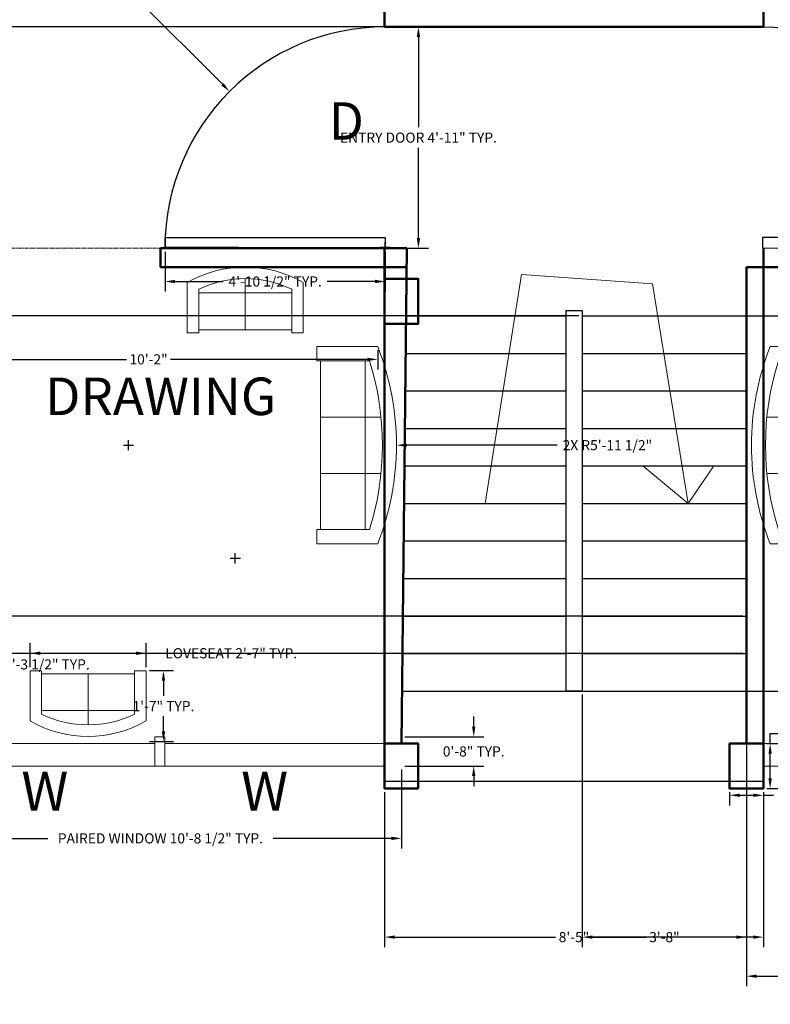
# Model space of a CAD drawing. Units: inches. Extents: x -15 to 796, y 111 to 651.
# Tile 2 of 6: x 216 to 416, y 111 to 373. Entities that reach past the tile are written whole.
import ezdxf

# ---------------------------------------------------------------- set-up
doc = ezdxf.new("R2010")
doc.units = ezdxf.units.IN
doc.header["$MEASUREMENT"] = 0
doc.linetypes.add('DASHED2', pattern=[0.375, 0.25, -0.125])
doc.layers.get('0').update_dxf_attribs({"color": 1})
for name, color, linetype, lineweight in [('A-ANNO-DIMS', 2, 'Continuous', 18), ('A-ANNO-SYMB', 2, 'Continuous', 18), ('A-ANNO-TEXT', 7, 'Continuous', 18), ('A-AREA-IDEN', 7, 'Continuous', 25), ('A-COLS', 1, 'Continuous', 50), ('A-DOOR', 3, 'Continuous', 25), ('A-FLOR-STRS', 7, 'Continuous', 25), ('A-FURN', 8, 'Continuous', 18), ('A-GLAZ', 4, 'Continuous', 18), ('A-WALL', 7, 'Continuous', 50), ('A-WALL-OVHD', 7, 'DASHED2', 18)]:
    doc.layers.add(name, color=color, linetype=linetype, lineweight=lineweight)
doc.styles.get("Standard").update_dxf_attribs({"font": 'arial.ttf'})
doc.dimstyles.get("Standard").update_dxf_attribs({"dimscale": 15, "dimtxt": 0.18, "dimasz": 0.18, "dimexe": 0.18, "dimexo": 0.0625, "dimgap": 0.09, "dimtad": 0, "dimtih": 1, "dimtoh": 1, "dimdec": 0, "dimzin": 0, "dimdsep": 46, "dimlunit": 3, "dimtxsty": 'Standard', "dimcen": 0.09, "dimadec": 0, "dimazin": 0, "dimtfac": 1, "dimtdec": 0, "dimtofl": 0, "dimtmove": 0, "dimatfit": 3, "dimfxl": 1, "dimtolj": 1, "dimtzin": 0, "dimarcsym": 0})

# ---------------------------------------------------------------- blocks, each defined once
blk = doc.blocks.new('Sofa - Roundback Loveseat 5 ft.')
for p, q in [((0, -32.44198), (0, -5.99998)), ((-24, -33.99998), (-24, -11.46958)), ((-23.9998, -13.38178), (23.99986, -13.38178)), ((24.00004, -33.99998), (24.00004, -11.46958)), ((-24, -32.44198), (24.00004, -32.44198))]:
    blk.add_line(p, q)
for points in [[(-24, -33.99998), (-30, -33.99998), (-30, -7.99998)], [(30.00004, -7.99998), (30.00004, -33.99998), (24.00004, -33.99998)]]:
    blk.add_lwpolyline(points)
for centre, radius, start, end in [((0, -60.24998), 60.24998, 60.13715, 119.8628), ((0, -61.38438), 55.38444, 64.32083, 115.6792)]:
    blk.add_arc(centre, radius, start, end)
blk = doc.blocks.new('Sofa - Roundback 7 ft.')
for p, q in [((-12.00002, -32.4421), (-12.00003, -6.5971)), ((11.99997, -32.4421), (11.99998, -6.5971)), ((-36.000027, -34), (-36.000027, -11.4696)), ((35.99998, -34), (35.99998, -11.4696)), ((-35.999844, -13.3819), (35.9998, -13.3819)), ((-36.000027, -32.4421), (35.99998, -32.4421))]:
    blk.add_line(p, q)
for points in [[(-36.000027, -34), (-42.000027, -34), (-42.000027, -8)], [(41.99998, -8), (41.99998, -34), (35.99998, -34)]]:
    blk.add_lwpolyline(points)
for centre, radius, start, end in [((0, -114.25), 114.25, 68.43141, 111.5686), ((-0.00001, -127.1968), 121.1968, 72.72033, 107.2797)]:
    blk.add_arc(centre, radius, start, end)
blk = doc.blocks.new('*D18')
at = {"layer": 'A-ANNO-DIMS', "color": 0, "lineweight": -2, "transparency": 16777216}
for p, q in [((409.68, 179.19), (409.68, 115.42)), ((697.18, 179.19), (697.18, 115.42)), ((412.38, 118.12), (539.23, 118.12)), ((694.48, 118.12), (567.64, 118.12))]:
    blk.add_line(p, q, dxfattribs=at)
at = {"layer": 'A-ANNO-DIMS', "color": 0, "transparency": 16777216}
for points in [[(412.38, 118.57), (412.38, 117.67), (409.68, 118.12)], [(694.48, 118.57), (694.48, 117.67), (697.18, 118.12)]]:
    blk.add_solid(points, dxfattribs=at)
at = {"layer": 'Defpoints', "color": 0, "transparency": 16777216}
for p in [(409.68, 180.13), (697.18, 180.13), (697.18, 118.12)]:
    blk.add_point(p, dxfattribs=at)
at = {"layer": 'A-ANNO-DIMS', "color": 0, "transparency": 16777216, "insert": (553.43, 118.12), "char_height": 2.7, "attachment_point": 5}
blk.add_mtext("\\A1;{\\H5.55556x;24'}", dxfattribs=at)
blk = doc.blocks.new('*D27')
at = {"layer": 'A-ANNO-DIMS', "color": 0, "lineweight": -2, "transparency": 16777216}
for p, q in [((189.18, 283.46), (189.18, 285.22)), ((311.36, 284.98), (311.36, 279.82)), ((191.88, 282.52), (244.41, 282.52)), ((308.66, 282.52), (256.13, 282.52))]:
    blk.add_line(p, q, dxfattribs=at)
at = {"layer": 'A-ANNO-DIMS', "color": 0, "transparency": 16777216}
for points in [[(191.88, 282.97), (191.88, 282.07), (189.18, 282.52)], [(308.66, 282.97), (308.66, 282.07), (311.36, 282.52)]]:
    blk.add_solid(points, dxfattribs=at)
at = {"layer": 'Defpoints', "color": 0, "transparency": 16777216}
for p in [(311.36, 285.92), (189.18, 282.52), (189.18, 282.52)]:
    blk.add_point(p, dxfattribs=at)
at = {"layer": 'A-ANNO-DIMS', "color": 0, "transparency": 16777216, "insert": (250.27, 282.52), "char_height": 2.7, "attachment_point": 5}
blk.add_mtext('\\A1;10\'-2"', dxfattribs=at)
blk = doc.blocks.new('DOOR-ENTRY-59IN')
blk.add_lwpolyline([(0, -0.29), (-58.71, 0), (-58.71, 2.57), (0, 2.57)], close=True)
blk.add_arc((0, 0), 58.71, 90, 180)
blk = doc.blocks.new('WIN-LIVING-PAIRED')
for p, q in [((0, 6), (62.78, 6)), ((62.78, 7.78), (65.45, 7.78)), ((62.78, 0), (62.78, 7.78)), ((65.45, 7.78), (65.45, 0)), ((65.45, 6), (128.5, 6)), ((4, 0), (124, 0)), ((65.45, 0), (62.78, 0))]:
    blk.add_line(p, q)
blk = doc.blocks.new('COL-9X12')
blk.add_lwpolyline([(9, 0), (0, 0), (0, 12), (9, 12)], close=True)
blk = doc.blocks.new('*D35')
at = {"layer": 'A-ANNO-DIMS', "color": 0, "lineweight": -2, "transparency": 16777216}
for p, q in [((415.98, 180.13), (415.98, 182.83)), ((415.98, 182.83), (418.68, 182.83)), ((415.12, 180.13), (418.68, 180.13)), ((415.98, 170.83), (415.98, 177.43)), ((415.12, 168.13), (418.68, 168.13))]:
    blk.add_line(p, q, dxfattribs=at)
at = {"layer": 'A-ANNO-DIMS', "color": 0, "transparency": 16777216}
for points in [[(415.53, 177.43), (416.43, 177.43), (415.98, 180.13)], [(415.53, 170.83), (416.43, 170.83), (415.98, 168.13)]]:
    blk.add_solid(points, dxfattribs=at)
at = {"layer": 'Defpoints', "color": 0, "transparency": 16777216}
for p in [(414.18, 180.13), (415.98, 180.13), (414.18, 168.13)]:
    blk.add_point(p, dxfattribs=at)
at = {"layer": 'A-ANNO-DIMS', "color": 0, "transparency": 16777216, "insert": (436.94, 182.83), "char_height": 2.7, "attachment_point": 5}
blk.add_mtext('\\A1;COLUMN 1\'-0" TYP.', dxfattribs=at)
blk = doc.blocks.new('*D36')
at = {"layer": 'A-ANNO-DIMS', "color": 0, "lineweight": -2, "transparency": 16777216}
for p, q in [((405.18, 167.19), (405.18, 163.63)), ((407.88, 166.33), (411.48, 166.33)), ((414.18, 167.19), (414.18, 163.63)), ((414.18, 166.33), (416.88, 166.33))]:
    blk.add_line(p, q, dxfattribs=at)
at = {"layer": 'A-ANNO-DIMS', "color": 0, "transparency": 16777216}
for points in [[(407.88, 166.78), (407.88, 165.88), (405.18, 166.33)], [(411.48, 166.78), (411.48, 165.88), (414.18, 166.33)]]:
    blk.add_solid(points, dxfattribs=at)
at = {"layer": 'Defpoints', "color": 0, "transparency": 16777216}
for p in [(405.18, 168.13), (414.18, 168.13), (414.18, 166.33)]:
    blk.add_point(p, dxfattribs=at)
at = {"layer": 'A-ANNO-DIMS', "color": 0, "transparency": 16777216, "insert": (426.46, 166.33), "char_height": 2.7, "attachment_point": 5}
blk.add_mtext('\\A1;0\'-9" TYP.', dxfattribs=at)
blk = doc.blocks.new('*D41')
at = {"layer": 'A-ANNO-DIMS', "color": 0, "lineweight": -2, "transparency": 16777216}
for p, q in [((218.67, 200.49), (218.67, 206.89)), ((249.6, 200.49), (249.6, 206.89)), ((221.37, 204.19), (246.9, 204.19)), ((249.6, 204.19), (252.3, 204.19))]:
    blk.add_line(p, q, dxfattribs=at)
at = {"layer": 'A-ANNO-DIMS', "color": 0, "transparency": 16777216}
for points in [[(221.37, 204.64), (221.37, 203.74), (218.67, 204.19)], [(246.9, 204.64), (246.9, 203.74), (249.6, 204.19)]]:
    blk.add_solid(points, dxfattribs=at)
at = {"layer": 'Defpoints', "color": 0, "transparency": 16777216}
for p in [(249.6, 204.19), (218.67, 199.55), (249.6, 199.55)]:
    blk.add_point(p, dxfattribs=at)
at = {"layer": 'A-ANNO-DIMS', "color": 0, "transparency": 16777216, "insert": (272.3, 204.19), "char_height": 2.7, "attachment_point": 5}
blk.add_mtext('\\A1;LOVESEAT 2\'-7" TYP.', dxfattribs=at)
blk = doc.blocks.new('*D42')
at = {"layer": 'A-ANNO-DIMS', "color": 0, "lineweight": -2, "transparency": 16777216}
for p, q in [((250.54, 199.55), (256.94, 199.55)), ((254.24, 196.85), (254.24, 192.8)), ((254.24, 183.35), (254.24, 187.39)), ((250.54, 180.65), (256.94, 180.65))]:
    blk.add_line(p, q, dxfattribs=at)
at = {"layer": 'A-ANNO-DIMS', "color": 0, "transparency": 16777216}
for points in [[(253.79, 196.85), (254.69, 196.85), (254.24, 199.55)], [(253.79, 183.35), (254.69, 183.35), (254.24, 180.65)]]:
    blk.add_solid(points, dxfattribs=at)
at = {"layer": 'Defpoints', "color": 0, "transparency": 16777216}
for p in [(249.6, 199.55), (249.6, 180.65), (254.24, 180.65)]:
    blk.add_point(p, dxfattribs=at)
at = {"layer": 'A-ANNO-DIMS', "color": 0, "transparency": 16777216, "insert": (254.24, 190.1), "char_height": 2.7, "attachment_point": 5}
blk.add_mtext('\\A1;1\'-7" TYP.', dxfattribs=at)
blk = doc.blocks.new('*D57')
at = {"layer": 'A-ANNO-DIMS', "color": 0, "lineweight": -2, "transparency": 16777216}
for p, q in [((314.31, 371.13), (324.92, 371.13)), ((322.22, 368.43), (322.22, 344.37)), ((322.22, 314.83), (322.22, 338.88)), ((314.31, 312.13), (324.92, 312.13))]:
    blk.add_line(p, q, dxfattribs=at)
at = {"layer": 'A-ANNO-DIMS', "color": 0, "transparency": 16777216}
for points in [[(321.77, 368.43), (322.67, 368.43), (322.22, 371.13)], [(321.77, 314.83), (322.67, 314.83), (322.22, 312.13)]]:
    blk.add_solid(points, dxfattribs=at)
at = {"layer": 'Defpoints', "color": 0, "transparency": 16777216}
for p in [(313.37, 371.13), (322.22, 371.13), (313.37, 312.13)]:
    blk.add_point(p, dxfattribs=at)
at = {"layer": 'A-ANNO-DIMS', "color": 0, "transparency": 16777216, "insert": (322.22, 341.63), "char_height": 2.7, "attachment_point": 5}
blk.add_mtext('\\A1;ENTRY DOOR 4\'-11" TYP.', dxfattribs=at)
blk = doc.blocks.new('*D58')
at = {"layer": 'A-ANNO-DIMS', "color": 0, "lineweight": -2, "transparency": 16777216}
for p, q in [((254.66, 311.19), (254.66, 300.58)), ((313.37, 311.19), (313.37, 300.58)), ((257.36, 303.28), (270.19, 303.28)), ((310.67, 303.28), (297.85, 303.28))]:
    blk.add_line(p, q, dxfattribs=at)
at = {"layer": 'A-ANNO-DIMS', "color": 0, "transparency": 16777216}
for points in [[(257.36, 303.73), (257.36, 302.83), (254.66, 303.28)], [(310.67, 303.73), (310.67, 302.83), (313.37, 303.28)]]:
    blk.add_solid(points, dxfattribs=at)
at = {"layer": 'Defpoints', "color": 0, "transparency": 16777216}
for p in [(254.66, 312.13), (313.37, 312.13), (313.37, 303.28)]:
    blk.add_point(p, dxfattribs=at)
at = {"layer": 'A-ANNO-DIMS', "color": 0, "transparency": 16777216, "insert": (284.02, 303.28), "char_height": 2.7, "attachment_point": 5}
blk.add_mtext('\\A1;4\'-10 1/2" TYP.', dxfattribs=at)
blk = doc.blocks.new('*D63')
at = {"layer": 'A-ANNO-DIMS', "color": 0, "lineweight": -2, "transparency": 16777216}
for p, q in [((189.18, 173.19), (189.18, 152.15)), ((317.68, 173.19), (317.68, 152.15)), ((191.88, 154.85), (223.38, 154.85)), ((314.98, 154.85), (283.48, 154.85))]:
    blk.add_line(p, q, dxfattribs=at)
at = {"layer": 'A-ANNO-DIMS', "color": 0, "transparency": 16777216}
for points in [[(191.88, 155.3), (191.88, 154.4), (189.18, 154.85)], [(314.98, 155.3), (314.98, 154.4), (317.68, 154.85)]]:
    blk.add_solid(points, dxfattribs=at)
at = {"layer": 'Defpoints', "color": 0, "transparency": 16777216}
for p in [(189.18, 174.13), (317.68, 174.13), (317.68, 154.85)]:
    blk.add_point(p, dxfattribs=at)
at = {"layer": 'A-ANNO-DIMS', "color": 0, "transparency": 16777216, "insert": (253.43, 154.85), "char_height": 2.7, "attachment_point": 5}
blk.add_mtext('\\A1;PAIRED WINDOW 10\'-8 1/2" TYP.', dxfattribs=at)
blk = doc.blocks.new('*D64')
at = {"layer": 'A-ANNO-DIMS', "color": 0, "lineweight": -2, "transparency": 16777216}
for p, q in [((336.96, 184.6), (336.96, 187.3)), ((318.62, 181.9), (339.66, 181.9)), ((318.62, 174.13), (339.66, 174.13)), ((336.96, 171.43), (336.96, 168.73))]:
    blk.add_line(p, q, dxfattribs=at)
at = {"layer": 'A-ANNO-DIMS', "color": 0, "transparency": 16777216}
for points in [[(336.51, 184.6), (337.41, 184.6), (336.96, 181.9)], [(336.51, 171.43), (337.41, 171.43), (336.96, 174.13)]]:
    blk.add_solid(points, dxfattribs=at)
at = {"layer": 'Defpoints', "color": 0, "transparency": 16777216}
for p in [(317.68, 181.9), (336.96, 181.9), (317.68, 174.13)]:
    blk.add_point(p, dxfattribs=at)
at = {"layer": 'A-ANNO-DIMS', "color": 0, "transparency": 16777216, "insert": (336.96, 178.02), "char_height": 2.7, "attachment_point": 5}
blk.add_mtext('\\A1;0\'-8" TYP.', dxfattribs=at)
blk = doc.blocks.new('*D66')
at = {"layer": 'A-ANNO-DIMS', "color": 0, "lineweight": -2, "transparency": 16777216}
for p, q in [((192.37, 199.77), (192.37, 203.92)), ((207.87, 199.77), (207.87, 203.92)), ((195.07, 201.22), (205.17, 201.22)), ((207.87, 201.22), (210.57, 201.22))]:
    blk.add_line(p, q, dxfattribs=at)
at = {"layer": 'A-ANNO-DIMS', "color": 0, "transparency": 16777216}
for points in [[(195.07, 201.67), (195.07, 200.77), (192.37, 201.22)], [(205.17, 201.67), (205.17, 200.77), (207.87, 201.22)]]:
    blk.add_solid(points, dxfattribs=at)
at = {"layer": 'Defpoints', "color": 0, "transparency": 16777216}
for p in [(207.87, 201.22), (192.37, 198.83), (207.87, 198.83)]:
    blk.add_point(p, dxfattribs=at)
at = {"layer": 'A-ANNO-DIMS', "color": 0, "transparency": 16777216, "insert": (223.17, 201.22), "char_height": 2.7, "attachment_point": 5}
blk.add_mtext('\\A1;1\'-3 1/2" TYP.', dxfattribs=at)
blk = doc.blocks.new('*D67')
at = {"layer": 'A-ANNO-DIMS', "color": 0, "lineweight": -2, "transparency": 16777216}
for p, q in [((313.19, 167.19), (313.19, 125.83)), ((414.18, 167.19), (414.18, 125.83)), ((315.89, 128.53), (358.75, 128.53)), ((411.48, 128.53), (368.63, 128.53))]:
    blk.add_line(p, q, dxfattribs=at)
at = {"layer": 'A-ANNO-DIMS', "color": 0, "transparency": 16777216}
for points in [[(315.89, 128.98), (315.89, 128.08), (313.19, 128.53)], [(411.48, 128.98), (411.48, 128.08), (414.18, 128.53)]]:
    blk.add_solid(points, dxfattribs=at)
at = {"layer": 'Defpoints', "color": 0, "transparency": 16777216}
for p in [(313.19, 168.13), (414.18, 168.13), (414.18, 128.53)]:
    blk.add_point(p, dxfattribs=at)
at = {"layer": 'A-ANNO-DIMS', "color": 0, "transparency": 16777216, "insert": (363.69, 128.53), "char_height": 2.7, "attachment_point": 5}
blk.add_mtext('\\A1;8\'-5"', dxfattribs=at)
blk = doc.blocks.new('*D68')
at = {"layer": 'A-ANNO-DIMS', "color": 0, "lineweight": -2, "transparency": 16777216}
for p, q in [((366.85, 294.11), (739.48, 294.11)), ((736.78, 291.41), (736.78, 246.84)), ((736.78, 196.81), (736.78, 241.38)), ((366.85, 194.11), (739.48, 194.11))]:
    blk.add_line(p, q, dxfattribs=at)
at = {"layer": 'A-ANNO-DIMS', "color": 0, "transparency": 16777216}
for points in [[(736.33, 291.41), (737.23, 291.41), (736.78, 294.11)], [(736.33, 196.81), (737.23, 196.81), (736.78, 194.11)]]:
    blk.add_solid(points, dxfattribs=at)
at = {"layer": 'Defpoints', "color": 0, "transparency": 16777216}
for p in [(365.91, 294.11), (736.78, 294.11), (365.91, 194.11)]:
    blk.add_point(p, dxfattribs=at)
at = {"layer": 'A-ANNO-DIMS', "color": 0, "transparency": 16777216, "insert": (736.78, 244.11), "char_height": 2.7, "attachment_point": 5}
blk.add_mtext('\\A1;8\'-4"', dxfattribs=at)
blk = doc.blocks.new('*D69')
at = {"layer": 'A-ANNO-DIMS', "color": 0, "lineweight": -2, "transparency": 16777216}
for p, q in [((-9.42, 214.11), (-9.42, 216.81)), ((-9.42, 216.81), (-6.72, 216.81)), ((408.74, 214.11), (-12.12, 214.11)), ((-9.42, 206.81), (-9.42, 211.41)), ((408.74, 204.11), (-12.12, 204.11))]:
    blk.add_line(p, q, dxfattribs=at)
at = {"layer": 'A-ANNO-DIMS', "color": 0, "transparency": 16777216}
for points in [[(-9.87, 211.41), (-8.97, 211.41), (-9.42, 214.11)], [(-9.87, 206.81), (-8.97, 206.81), (-9.42, 204.11)]]:
    blk.add_solid(points, dxfattribs=at)
at = {"layer": 'Defpoints', "color": 0, "transparency": 16777216}
for p in [(-9.42, 214.11), (409.68, 214.11), (409.68, 204.11)]:
    blk.add_point(p, dxfattribs=at)
at = {"layer": 'A-ANNO-DIMS', "color": 0, "transparency": 16777216, "insert": (-0.73, 216.81), "char_height": 2.7, "attachment_point": 5}
blk.add_mtext('\\A1;0\'-10"', dxfattribs=at)
blk = doc.blocks.new('*D73')
at = {"layer": 'A-ANNO-DIMS', "color": 0, "lineweight": -2, "transparency": 16777216}
for p, q in [((365.91, 193.17), (365.91, 125.83)), ((409.68, 193.17), (409.68, 125.83)), ((368.61, 128.53), (382.86, 128.53)), ((406.98, 128.53), (392.73, 128.53))]:
    blk.add_line(p, q, dxfattribs=at)
at = {"layer": 'A-ANNO-DIMS', "color": 0, "transparency": 16777216}
for points in [[(368.61, 128.98), (368.61, 128.08), (365.91, 128.53)], [(406.98, 128.98), (406.98, 128.08), (409.68, 128.53)]]:
    blk.add_solid(points, dxfattribs=at)
at = {"layer": 'Defpoints', "color": 0, "transparency": 16777216}
for p in [(365.91, 194.11), (409.68, 194.11), (409.68, 128.53)]:
    blk.add_point(p, dxfattribs=at)
at = {"layer": 'A-ANNO-DIMS', "color": 0, "transparency": 16777216, "insert": (387.8, 128.53), "char_height": 2.7, "attachment_point": 5}
blk.add_mtext('\\A1;3\'-8"', dxfattribs=at)
blk = doc.blocks.new('*D74')
at = {"layer": 'A-ANNO-DIMS', "color": 0, "lineweight": -2, "transparency": 16777216}
for p, q in [((413.24, 371.13), (-12.12, 371.13)), ((-9.42, 368.43), (-9.42, 335.35)), ((-9.42, 296.81), (-9.42, 329.89)), ((364.97, 294.11), (-12.12, 294.11))]:
    blk.add_line(p, q, dxfattribs=at)
at = {"layer": 'A-ANNO-DIMS', "color": 0, "transparency": 16777216}
for points in [[(-9.87, 368.43), (-8.97, 368.43), (-9.42, 371.13)], [(-9.87, 296.81), (-8.97, 296.81), (-9.42, 294.11)]]:
    blk.add_solid(points, dxfattribs=at)
at = {"layer": 'Defpoints', "color": 0, "transparency": 16777216}
for p in [(414.18, 371.13), (-9.42, 294.11), (365.91, 294.11)]:
    blk.add_point(p, dxfattribs=at)
at = {"layer": 'A-ANNO-DIMS', "color": 0, "transparency": 16777216, "insert": (-9.42, 332.62), "char_height": 2.7, "attachment_point": 5}
blk.add_mtext('\\A1;6\'-5"', dxfattribs=at)
blk = doc.blocks.new('*D81')
at = {"layer": 'A-ANNO-DIMS', "color": 0, "lineweight": -2, "transparency": 16777216}
for p, q in [((410.62, 194.11), (739.48, 194.11)), ((736.78, 191.41), (736.78, 183.82)), ((736.78, 170.83), (736.78, 178.41)), ((415.12, 168.13), (739.48, 168.13))]:
    blk.add_line(p, q, dxfattribs=at)
at = {"layer": 'A-ANNO-DIMS', "color": 0, "transparency": 16777216}
for points in [[(736.33, 191.41), (737.23, 191.41), (736.78, 194.11)], [(736.33, 170.83), (737.23, 170.83), (736.78, 168.13)]]:
    blk.add_solid(points, dxfattribs=at)
at = {"layer": 'Defpoints', "color": 0, "transparency": 16777216}
for p in [(409.68, 194.11), (414.18, 168.13), (736.78, 168.13)]:
    blk.add_point(p, dxfattribs=at)
at = {"layer": 'A-ANNO-DIMS', "color": 0, "transparency": 16777216, "insert": (736.78, 181.12), "char_height": 2.7, "attachment_point": 5}
blk.add_mtext('\\A1;2\'-2"', dxfattribs=at)
blk = doc.blocks.new('*D84')
at = {"layer": 'A-ANNO-DIMS', "color": 0, "lineweight": -2, "transparency": 16777216}
for p, q in [((161.25, 229.5), (194.88, 229.5)), ((272.04, 229.5), (274.74, 229.5)), ((273.39, 228.15), (273.39, 230.85))]:
    blk.add_line(p, q, dxfattribs=at)
at = {"layer": 'A-ANNO-DIMS', "color": 0, "transparency": 16777216}
blk.add_solid([(194.88, 229.95), (194.88, 229.05), (197.58, 229.5)], dxfattribs=at)
at = {"layer": 'Defpoints', "color": 0, "transparency": 16777216}
for p in [(197.58, 229.5), (273.39, 229.5)]:
    blk.add_point(p, dxfattribs=at)
at = {"layer": 'A-ANNO-DIMS', "color": 0, "transparency": 16777216, "insert": (152.09, 229.5), "char_height": 2.7, "attachment_point": 5}
blk.add_mtext('\\A1;2X R6\'-4"', dxfattribs=at)
blk = doc.blocks.new('*D85')
at = {"layer": 'A-ANNO-DIMS', "color": 0, "lineweight": -2, "transparency": 16777216}
for p, q in [((244.9, 258.3), (244.9, 261)), ((243.55, 259.65), (246.25, 259.65)), ((359.24, 259.65), (319.06, 259.65))]:
    blk.add_line(p, q, dxfattribs=at)
at = {"layer": 'A-ANNO-DIMS', "color": 0, "transparency": 16777216}
blk.add_solid([(319.06, 260.1), (319.06, 259.2), (316.36, 259.65)], dxfattribs=at)
at = {"layer": 'Defpoints', "color": 0, "transparency": 16777216}
for p in [(244.9, 259.65), (316.36, 259.65)]:
    blk.add_point(p, dxfattribs=at)
at = {"layer": 'A-ANNO-DIMS', "color": 0, "transparency": 16777216, "insert": (372.59, 259.65), "char_height": 2.7, "attachment_point": 5}
blk.add_mtext('\\A1;2X R5\'-11 1/2"', dxfattribs=at)
blk = doc.blocks.new('*D88')
at = {"layer": 'A-ANNO-DIMS', "color": 0, "lineweight": -2, "transparency": 16777216}
for p, q in [((244.25, 378.84), (246.95, 378.84)), ((246.95, 378.84), (269.95, 355.84)), ((312.02, 312.41), (314.72, 312.41)), ((313.37, 311.06), (313.37, 313.76))]:
    blk.add_line(p, q, dxfattribs=at)
at = {"layer": 'A-ANNO-DIMS', "color": 0, "transparency": 16777216}
blk.add_solid([(270.27, 356.16), (269.63, 355.52), (271.86, 353.93)], dxfattribs=at)
at = {"layer": 'Defpoints', "color": 0, "transparency": 16777216}
for p in [(271.86, 353.93), (313.37, 312.41)]:
    blk.add_point(p, dxfattribs=at)
at = {"layer": 'A-ANNO-DIMS', "color": 0, "transparency": 16777216, "insert": (233.82, 378.84), "char_height": 2.7, "attachment_point": 5}
blk.add_mtext('\\A1;R4\'-10 1/2"', dxfattribs=at)

msp = doc.modelspace()

# ---------------------------------------------------------------- linework, layer by layer
at = {"layer": 'A-ANNO-SYMB'}
for p, q in [((339.99, 244.11), (349.68, 305.13)), ((349.68, 305.13), (384.62, 302.63)), ((384.62, 302.63), (394.11, 244.11)), ((394.11, 244.11), (382, 254.11)), ((382, 254.11), (401.01, 254.11)), ((401.01, 254.11), (394.11, 244.11))]:
    msp.add_line(p, q, dxfattribs=at)
at = {"layer": 'A-FLOR-STRS'}
for p, q in [((318.91, 294.11), (361.6, 294.11)), ((365.91, 294.11), (414.18, 294.11)), ((318.8, 284.11), (361.6, 284.11)), ((365.91, 284.11), (409.68, 284.11)), ((318.69, 274.11), (361.6, 274.11)), ((365.91, 274.11), (409.68, 274.11)), ((318.59, 264.11), (361.6, 264.11)), ((365.91, 264.11), (409.68, 264.11)), ((318.48, 254.11), (361.6, 254.11)), ((365.91, 254.11), (409.68, 254.11)), ((318.37, 244.11), (361.6, 244.11)), ((365.91, 244.11), (409.68, 244.11)), ((318.26, 234.11), (361.6, 234.11)), ((365.91, 234.11), (409.68, 234.11)), ((318.16, 224.11), (361.6, 224.11)), ((365.91, 224.11), (409.68, 224.11)), ((318.05, 214.11), (361.6, 214.11)), ((365.91, 214.11), (409.68, 214.11)), ((317.94, 204.11), (361.6, 204.11)), ((365.91, 204.11), (409.68, 204.11)), ((317.83, 194.11), (409.68, 194.11)), ((313.18, 170.11), (414.18, 170.11))]:
    msp.add_line(p, q, dxfattribs=at)
msp.add_lwpolyline([(361.6, 295.57), (365.91, 295.57), (365.91, 194.11), (361.6, 194.11)], close=True, dxfattribs=at)
at = {"layer": 'A-GLAZ'}
msp.add_line((414.18, 174.13), (504.18, 174.13), dxfattribs=at)
at = {"layer": 'A-WALL'}
for p, q in [((414.18, 371.13), (414.18, 598.13)), ((313.18, 371.13), (313.18, 589.13)), ((313.18, 374.68), (313.18, 371.13)), ((414.18, 371.13), (414.18, 374.68)), ((313.18, 371.13), (319.74, 371.13)), ((319.74, 371.13), (313.18, 371.13)), ((313.18, 371.13), (414.18, 371.13)), ((313.37, 371.13), (319.74, 371.13)), ((410.29, 371.1), (413.99, 371.13)), ((319.1, 312.13), (253.43, 312.13)), ((253.43, 307.13), (253.43, 312.13)), ((313.18, 174.13), (313.18, 312.13)), ((313.18, 312.13), (319.1, 312.13)), ((319.1, 312.13), (317.68, 180.13)), ((414.18, 168.13), (414.18, 312.13)), ((319.05, 307.13), (253.43, 307.13)), ((409.68, 307.13), (473.93, 307.13)), ((409.68, 284.11), (409.68, 307.13)), ((409.68, 284.11), (409.68, 292.01)), ((409.68, 180.13), (409.68, 284.11)), ((409.68, 180.13), (409.68, 274.11))]:
    msp.add_line(p, q, dxfattribs=at)
at = {"layer": 'A-WALL-OVHD'}
msp.add_line((253.43, 312.13), (189.18, 312.13), dxfattribs=at)

# ---------------------------------------------------------------- block references
at = {"layer": 'A-COLS', "rotation": 180}
msp.add_blockref('COL-9X12', (322.18, 304.01), dxfattribs=at)
at = {"layer": 'A-COLS', "extrusion": (0, 0, -1), "zscale": -1, "rotation": 180}
msp.add_blockref('COL-9X12', (-313.18, 304.01), dxfattribs=at)
at = {"layer": 'A-COLS'}
for p in [(313.19, 168.13), (405.18, 168.13)]:
    msp.add_blockref('COL-9X12', p, dxfattribs=at)
at = {"layer": 'A-DOOR'}
msp.add_blockref('DOOR-ENTRY-59IN', (313.37, 312.41), dxfattribs=at)
at = {"layer": 'A-DOOR', "extrusion": (0, 0, -1), "zscale": -1}
msp.add_blockref('DOOR-ENTRY-59IN', (-413.99, 312.41), dxfattribs=at)
at = {"layer": 'A-FURN', "xscale": -0.5154795599651856, "yscale": 0.5154795599651856, "zscale": 0.5154795599651856}
msp.add_blockref('Sofa - Roundback Loveseat 5 ft.', (276.05, 307.13), dxfattribs=at)
at = {"layer": 'A-FURN'}
for name, p, xscale, yscale, zscale, rotation in [('Sofa - Roundback 7 ft.', (316.36, 259.65), 0.6255113727593298, 0.6255113727593298, 0.6255113727593298, 270), ('Sofa - Roundback 7 ft.', (411, 259.65), -0.6255113727593298, 0.6255113727593298, 0.6255113727593298, 90), ('Sofa - Roundback Loveseat 5 ft.', (234.14, 182.02), -0.5154795599651856, 0.5154795599651856, 0.5154795599651856, 180)]:
    msp.add_blockref(name, p, dxfattribs=dict(at, xscale=xscale, yscale=yscale, zscale=zscale, rotation=rotation))
at = {"layer": 'A-GLAZ'}
msp.add_blockref('WIN-LIVING-PAIRED', (189.18, 174.13), dxfattribs=at)
at = {"layer": 'A-GLAZ', "extrusion": (0, 0, -1), "zscale": -1}
msp.add_blockref('WIN-LIVING-PAIRED', (-538.18, 174.13), dxfattribs=at)

# ---------------------------------------------------------------- texts
at = {"layer": 'A-ANNO-TEXT', "attachment_point": 1}
for s, width, gutter_width, insert, char_height in [('D', 13.2435, 1, (298.29, 351.05), 10), ('W', 19.9719, 52.27, (216.36, 172.64), 10.45), ('W', 19.9719, 52.27, (274.96, 172.64), 10.45)]:
    msp.add_mtext_dynamic_manual_height_columns(s, width=width, gutter_width=gutter_width, heights=[0], dxfattribs=dict(at, insert=insert, char_height=char_height))
at = {"layer": 'A-AREA-IDEN', "insert": (222.7, 277.67), "char_height": 10, "attachment_point": 1}
msp.add_mtext_dynamic_manual_height_columns('DRAWING', width=67.6028, gutter_width=50, heights=[0], dxfattribs=at)

# ---------------------------------------------------------------- dimensions: what is measured, and where the dimension line sits
at = {"layer": 'A-ANNO-DIMS'}
dim = msp.add_radius_dim(center=(313.37, 312.41), mpoint=(271.86, 353.93), dimstyle='Standard', override={"dimdec": 1, "dimlfac": 1, "dimrnd": 0, "dimzin": 1, "dimdsep": 46, "dimlunit": 4, "dimfrac": 2}, dxfattribs=at)
dim.commit()
dim.dimension.update_dxf_attribs({"geometry": '*D88', "text_midpoint": (233.82, 378.84), "dimtype": 164})
for base, p1, p2, picture, middle in [((-9.42, 294.11), (414.18, 371.13), (365.91, 294.11), '*D74', (-9.42, 332.62)), ((736.78, 294.11), (365.91, 194.11), (365.91, 294.11), '*D68', (736.78, 244.11)), ((-9.42, 214.11), (409.68, 204.11), (409.68, 214.11), '*D69', (-0.73, 216.81)), ((736.78, 168.13), (409.68, 194.11), (414.18, 168.13), '*D81', (736.78, 181.12))]:
    dim = msp.add_linear_dim(base=base, p1=p1, p2=p2, angle=90, dimstyle='Standard', override={"dimdec": 1, "dimlfac": 1, "dimrnd": 0, "dimzin": 1, "dimdsep": 46, "dimlunit": 4, "dimfrac": 2}, dxfattribs=at)
    dim.commit()
    dim.dimension.update_dxf_attribs({"geometry": picture, "text_midpoint": middle})
for base, p1, p2, angle, text, picture, middle in [((322.22, 371.13), (313.37, 312.13), (313.37, 371.13), 90, 'ENTRY DOOR <> TYP.', '*D57', (322.22, 341.63)), ((254.24, 180.65), (249.6, 199.55), (249.6, 180.65), 270, '<> TYP.', '*D42', (254.24, 190.1)), ((415.98, 180.13), (414.18, 168.13), (414.18, 180.13), 90, 'COLUMN <> TYP.', '*D35', (436.94, 182.83)), ((336.96, 181.9), (317.68, 174.13), (317.68, 181.9), 90, '<> TYP.', '*D64', (336.96, 178.02))]:
    dim = msp.add_linear_dim(base=base, p1=p1, p2=p2, angle=angle, text=text, dimstyle='Standard', override={"dimdec": 1, "dimlfac": 1, "dimrnd": 0, "dimzin": 1, "dimdsep": 46, "dimlunit": 4, "dimfrac": 2}, dxfattribs=at)
    dim.commit()
    dim.dimension.update_dxf_attribs({"geometry": picture, "text_midpoint": middle})
for base, p1, p2, text, override, picture, middle in [((313.37, 303.28), (254.66, 312.13), (313.37, 312.13), '<> TYP.', {"dimdec": 1, "dimlfac": 1, "dimrnd": 0, "dimzin": 1, "dimdsep": 46, "dimlunit": 4, "dimfrac": 2}, '*D58', (284.02, 303.28)), ((249.6, 204.19), (218.67, 199.55), (249.6, 199.55), 'LOVESEAT <> TYP.', {"dimdec": 1, "dimlfac": 1, "dimrnd": 0, "dimzin": 1, "dimdsep": 46, "dimlunit": 4, "dimfrac": 2}, '*D41', (272.3, 204.19)), ((207.87, 201.22), (192.37, 198.83), (207.87, 198.83), '<> TYP.', {"dimdec": 1, "dimlfac": 1, "dimrnd": 0, "dimzin": 1, "dimdsep": 46, "dimlunit": 4, "dimfrac": 2}, '*D66', (223.17, 201.22)), ((697.18184818, 118.12009751), (409.68184818, 180.12661683), (697.18184818, 180.12661683), '{\\H5.55556x;<>}', {"dimclrd": 0, "dimclre": 0, "dimclrt": 0}, '*D18', (553.43184818, 118.12009751)), ((317.68, 154.85), (189.18, 174.13), (317.68, 174.13), 'PAIRED WINDOW <> TYP.', {"dimdec": 1, "dimlfac": 1, "dimrnd": 0, "dimzin": 1, "dimdsep": 46, "dimlunit": 4, "dimfrac": 2}, '*D63', (253.43, 154.85)), ((414.18, 166.33), (405.18, 168.13), (414.18, 168.13), '<> TYP.', {"dimdec": 1, "dimlfac": 1, "dimrnd": 0, "dimzin": 1, "dimdsep": 46, "dimlunit": 4, "dimfrac": 2}, '*D36', (426.46, 166.33))]:
    dim = msp.add_linear_dim(base=base, p1=p1, p2=p2, text=text, dimstyle='Standard', override=override, dxfattribs=at)
    dim.commit()
    dim.dimension.update_dxf_attribs({"geometry": picture, "text_midpoint": middle})
for base, p1, p2, override, picture, middle in [((189.18, 282.52), (311.36, 285.92), (189.18, 282.52), {"dimclrd": 0, "dimclre": 0, "dimclrt": 0}, '*D27', (250.27, 282.52)), ((409.68, 128.53), (365.91, 194.11), (409.68, 194.11), {"dimdec": 1, "dimlfac": 1, "dimrnd": 0, "dimzin": 1, "dimdsep": 46, "dimlunit": 4, "dimfrac": 2}, '*D73', (387.8, 128.53)), ((414.18, 128.53), (313.19, 168.13), (414.18, 168.13), {"dimdec": 1, "dimlfac": 1, "dimrnd": 0, "dimzin": 1, "dimdsep": 46, "dimlunit": 4, "dimfrac": 2}, '*D67', (363.69, 128.53))]:
    dim = msp.add_linear_dim(base=base, p1=p1, p2=p2, dimstyle='Standard', override=override, dxfattribs=at)
    dim.commit()
    dim.dimension.update_dxf_attribs({"geometry": picture, "text_midpoint": middle})
for center, mpoint, picture, middle in [((244.9, 259.65), (316.36, 259.65), '*D85', (359.24, 259.65)), ((273.39, 229.5), (197.58, 229.5), '*D84', (152.09, 229.5))]:
    dim = msp.add_radius_dim(center=center, mpoint=mpoint, text='2X <>', dimstyle='Standard', override={"dimdec": 1, "dimlfac": 1, "dimrnd": 0, "dimzin": 1, "dimdsep": 46, "dimlunit": 4, "dimfrac": 2}, dxfattribs=at)
    dim.commit()
    dim.dimension.update_dxf_attribs({"geometry": picture, "text_midpoint": middle, "dimtype": 164})

doc.saveas('drawing.dxf')
